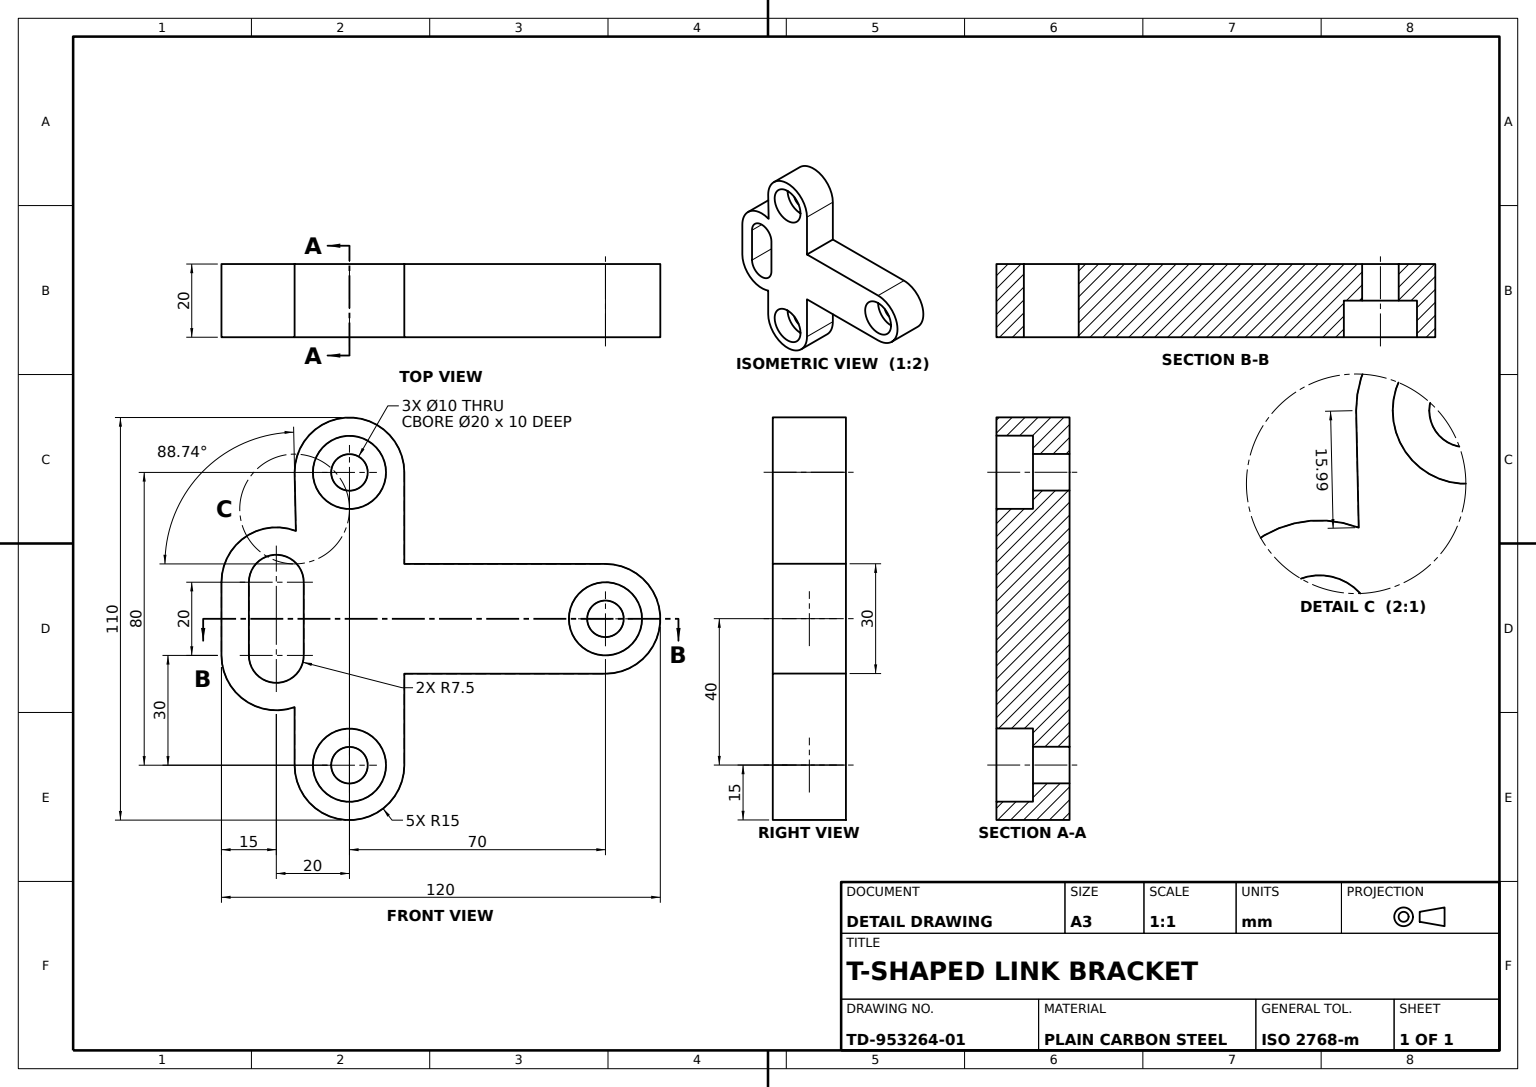
from build123d import *

# Parameters (mm, degrees)
T_BRACKET_PLATE_20MM_DEPTH     = 20
POCKET_A_SKETCH_R              = 10
TRIANGULAR_POCKET_A_10MM_DEPTH = 10
POCKET_B_SKETCH_R              = 5
TRIANGULAR_POCKET_B_10MM_DEPTH = 10


with BuildPart() as part:
    # T Profile Sketch → T Bracket Plate 20mm (new body)
    with BuildSketch(Plane.XY):
        with BuildLine():
            ThreePointArc((-14.647668653, 24.012585384), (-28.506322055, 22.354856741), (-35, 10))
            Line((-35, 10), (-35, -10))
            ThreePointArc((-35, -10), (-28.660254038, -22.247448714), (-15, -24.142135624))
            Line((-15, -24.142135624), (-15, -40))
            ThreePointArc((-15, -40), (0, -55), (15, -40))
            Line((15, -40), (15, -15))
            Line((15, -15), (70, -15))
            ThreePointArc((70, -15), (85, 0), (70, 15))
            Line((70, 15), (15, 15))
            Line((15, 15), (15, 40))
            ThreePointArc((15, 40), (0, 55), (-15, 40))
            Line((-15, 40), (-14.985436811, 39.339179624))
            Line((-14.985436811, 39.339179624), (-14.647668653, 24.012585384))
        make_face()
        with BuildLine():
            Line((-27.5, -10), (-27.5, 10))
            ThreePointArc((-27.5, 10), (-20, 17.5), (-12.5, 10))
            Line((-12.5, 10), (-12.5, -10))
            ThreePointArc((-12.5, -10), (-20, -17.5), (-27.5, -10))
        make_face(mode=Mode.SUBTRACT)
    extrude(amount=T_BRACKET_PLATE_20MM_DEPTH)

    # Pocket A Sketch → Triangular Pocket A 10mm (cut)
    with BuildSketch(Plane.XY.offset(20)):
        with Locations((0, 40)):
            Circle(POCKET_A_SKETCH_R)
        with Locations((0, -40)):
            Circle(POCKET_A_SKETCH_R)
        with Locations((70, 0)):
            Circle(POCKET_A_SKETCH_R)
    extrude(amount=-TRIANGULAR_POCKET_A_10MM_DEPTH, mode=Mode.SUBTRACT)

    # Pocket B Sketch → Triangular Pocket B 10mm (cut)
    with BuildSketch(Plane.XY.offset(10)):
        with Locations((0, 40)):
            Circle(POCKET_B_SKETCH_R)
        with Locations((0, -40)):
            Circle(POCKET_B_SKETCH_R)
        with Locations((70, 0)):
            Circle(POCKET_B_SKETCH_R)
    extrude(amount=-TRIANGULAR_POCKET_B_10MM_DEPTH, mode=Mode.SUBTRACT)


solid = part.part
